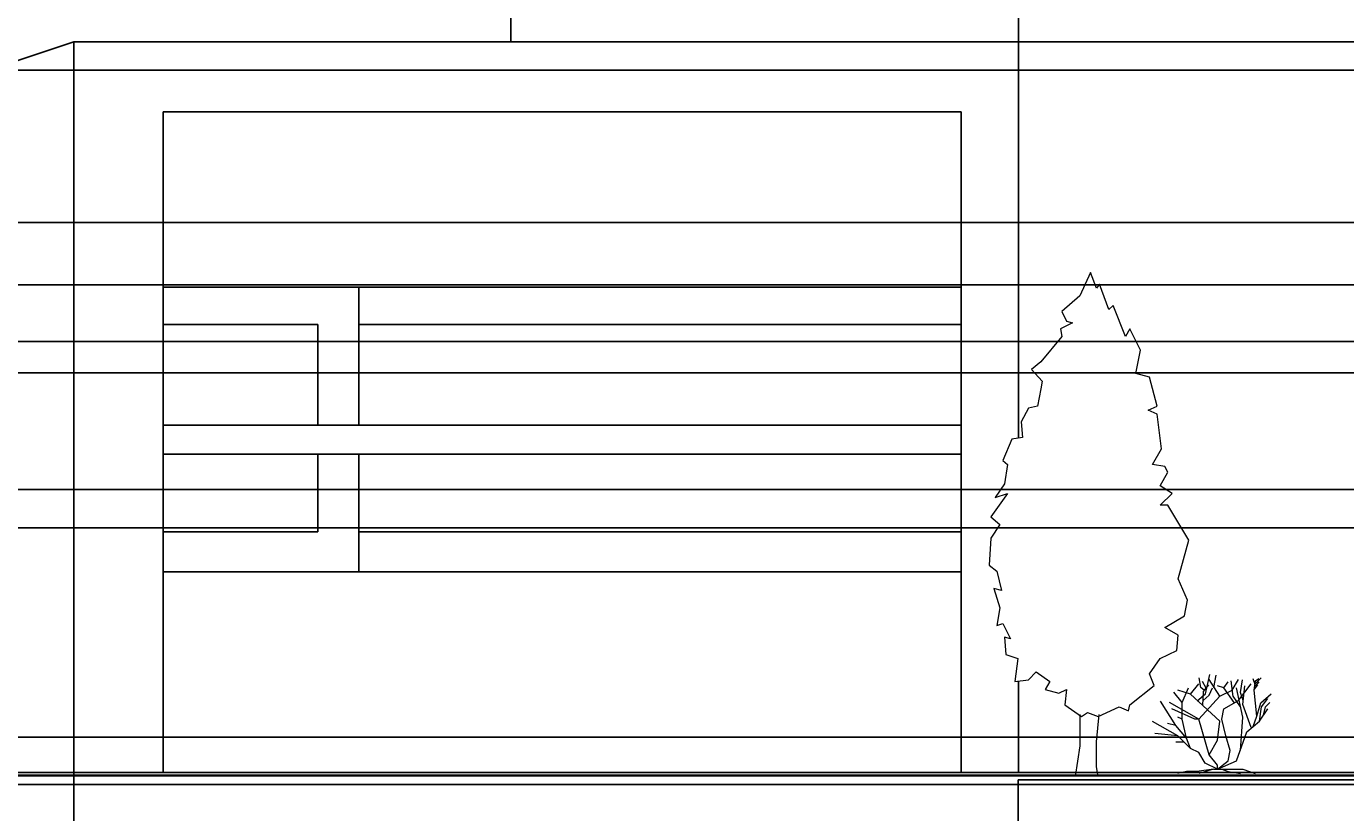
# Model space of a CAD drawing. Units: inches. Extents: x -32109 to 33221, y -19197 to 7608.
# Tile 21 of 25: x 15375 to 19011, y -2226 to -59. Entities that reach past the tile are written whole.
import ezdxf

# ---------------------------------------------------------------- set-up
doc = ezdxf.new("R2010")
doc.units = ezdxf.units.IN
doc.header["$MEASUREMENT"] = 0
for name, color, linetype, lineweight in [('A-ANNO-DIMS', 2, 'Continuous', 18), ('A-ELEV', 7, 'Continuous', 25), ('L-PLNT', 3, 'Continuous', 13)]:
    doc.layers.add(name, color=color, linetype=linetype, lineweight=lineweight)
doc.styles.get("Standard").update_dxf_attribs({"font": 'arial.ttf'})
doc.dimstyles.get("Standard").update_dxf_attribs({"dimtxt": 0.18, "dimasz": 0.18, "dimexe": 0.18, "dimexo": 0.0625, "dimgap": 0.09, "dimtad": 0, "dimtih": 1, "dimtoh": 1, "dimdec": 4, "dimzin": 0, "dimdsep": 46, "dimtxsty": 'Standard', "dimcen": 0.09, "dimadec": 0, "dimazin": 0, "dimtfac": 1, "dimtdec": 4, "dimtofl": 0, "dimtmove": 0, "dimatfit": 3, "dimfxl": 1, "dimtolj": 1, "dimtzin": 0, "dimarcsym": 0})

# ---------------------------------------------------------------- blocks, each defined once
blk = doc.blocks.new('*U2')
blk.add_lwpolyline([(-2.754, 191.699), (-6.78, 182.851), (-13.682, 176.953), (-11.956, 173.266), (-9.656, 172.529), (-14.257, 170.317), (-13.682, 167.368), (-21.733, 157.783), (-25.184, 154.834), (-21.158, 150.41), (-21.733, 147.461), (-22.884, 140.825), (-26.334, 140.087), (-29.21, 134.926), (-28.635, 129.028), (-32.661, 128.291), (-36.111, 120.18), (-34.386, 118.706), (-35.536, 111.333), (-38.987, 106.171), (-34.386, 107.646), (-40.712, 98.798), (-37.261, 95.849), (-40.712, 90.688), (-41.287, 80.366), (-38.412, 78.154), (-36.686, 70.781), (-39.562, 71.518), (-37.261, 64.145), (-38.412, 57.509), (-36.111, 58.247), (-33.236, 52.348), (-35.536, 53.086), (-34.961, 46.45), (-30.36, 44.975), (-31.51, 36.128), (-26.334, 36.865), (-23.459, 39.814), (-18.283, 36.128), (-20.008, 33.178), (-14.832, 31.704), (-11.956, 33.178), (-12.531, 27.28), (-6.205, 22.856), (-3.905, 24.331), (0.121, 22.856), (8.173, 26.543), (11.624, 25.068), (12.199, 27.28), (21.4, 34.653), (19.675, 39.077), (23.701, 44.975), (30.027, 47.924), (30.602, 53.823), (25.426, 56.772), (32.903, 61.196), (34.053, 67.094), (30.602, 75.205), (34.628, 89.951), (26.576, 103.222), (23.701, 103.222), (28.302, 107.646), (23.701, 110.595), (26.576, 115.756), (25.426, 117.968), (20.825, 118.706), (24.276, 124.604), (22.551, 137.876), (19.1, 139.35), (22.551, 140.825), (19.675, 151.884), (14.499, 153.359), (16.224, 162.207), (12.199, 170.317), (10.473, 167.368), (5.872, 179.165), (4.147, 177.69), (0.696, 187.275), (-0.454, 185.8)], close=True)
for points in [[(-6.813, 23.669), (-6.813, 11.669), (-8.627, 0)], [(0.387, 23.669), (-0.576, 13.271), (-0.576, 3.686), (0, 0)]]:
    blk.add_lwpolyline(points)
blk = doc.blocks.new('*U3')
for p, q in [((-12.471, 19.775), (-12.898, 22.044)), ((-11.433, 18.289), (-10.457, 22.749)), ((-8.16, 17.76), (-10.56, 21.6)), ((-9.48, 19.775), (-8.992, 22.592)), ((-5.086, 17.741), (-5.513, 21.34)), ((-5.28, 19.2), (-3.84, 21.6)), ((-3.377, 18.602), (-2.888, 21.575)), ((-0.508, 21.888), (-0.081, 20.558)), ((-0.203, 19.149), (0.102, 21.34)), ((0.041, 20.714), (1.384, 22.044)), ((0.102, 21.34), (0.835, 21.888)), ((-16.8, 16.32), (-18.72, 18.72)), ((-14.88, 18.24), (-17.76, 19.2)), ((-16.8, 16.32), (-15.36, 19.68)), ((-14.88, 18.24), (-12.96, 20.64)), ((-8.16, 12), (-14.88, 18.24)), ((-13.325, 16.724), (-11.433, 18.289)), ((-11.677, 19.071), (-12.471, 19.775)), ((-11.28, 19.619), (-12.104, 21.184)), ((-12.043, 15.628), (-11.921, 18.836)), ((-11.921, 18.836), (-10.64, 20.401)), ((-10.579, 18.054), (-9.846, 19.697)), ((-7.2, 19.68), (-8.64, 20.16)), ((-8.16, 17.76), (-5.28, 19.2)), ((-7.2, 19.68), (-6.24, 21.12)), ((-4.8, 16.32), (-7.2, 19.68)), ((-2.88, 12.96), (-4.32, 19.68)), ((-3.84, 16.8), (-0.96, 20.64)), ((-2.766, 16.802), (-3.377, 18.602)), ((-2.88, 15.84), (-2.4, 20.16)), ((0.346, 13.203), (-0.203, 19.149)), ((-0.142, 19.384), (0.59, 20.401)), ((-0.02, 20.01), (0.896, 21.105)), ((1.323, 16.254), (3.642, 18.289)), ((-18.24, 11.04), (-21.755, 16.655)), ((-12.96, 12.48), (-19.68, 16.32)), ((-16.8, 12.48), (-16.8, 16.32)), ((-12.96, 12.48), (-8.16, 17.76)), ((-11.982, 16.802), (-10.579, 18.054)), ((-7.2, 14.88), (-3.84, 16.8)), ((-3.377, 15.315), (-5.086, 17.819)), ((-0.96, 10.56), (-2.88, 15.84)), ((0.346, 13.203), (1.323, 16.254)), ((0.96, 12), (1.44, 15.36)), ((1.44, 15.36), (2.88, 17.28)), ((1.92, 13.44), (2.4, 15.36)), ((2.4, 15.36), (3.36, 16.32)), ((-13.92, 12.48), (-19.2, 14.88)), ((-16.8, 12.48), (-17.76, 12.96)), ((-15.84, 8.16), (-16.8, 12.48)), ((-12.96, 12.48), (-13.92, 12.48)), ((-10.56, 4.32), (-12.96, 12.48)), ((-7.68, 12.48), (-7.2, 14.88)), ((-6.72, 8.64), (-7.68, 12.48)), ((-3.36, 5.28), (-2.88, 12.96)), ((-0.48, 10.8), (0.346, 13.203)), ((0.96, 12), (2.88, 14.88)), ((-17.76, 8.64), (-23.663, 11.961)), ((-17.76, 8.64), (-23.128, 9.222)), ((-18.24, 11.04), (-20.16, 11.52)), ((-15.84, 8.16), (-18.24, 11.04)), ((-8.64, 7.68), (-8.16, 12)), ((-4.32, 2.88), (-1.92, 9.6)), ((-1.92, 9.6), (0.96, 12)), ((-16.32, 7.2), (-18.24, 7.2)), ((-14.88, 5.76), (-17.76, 8.64)), ((-14.88, 5.76), (-15.84, 8.16)), ((-10.56, 4.32), (-8.64, 7.68)), ((-5.76, 5.28), (-6.72, 8.64)), ((-12.96, 4.8), (-14.88, 5.76)), ((-11.52, 2.4), (-12.96, 4.8)), ((-8.64, 1.92), (-10.56, 4.32)), ((-6.24, 2.88), (-5.76, 5.28)), ((-15.84, 0.48), (-17.76, 0)), ((-13.44, 0.48), (-15.84, 0.48)), ((-9.6, 0.96), (-13.44, 0.48)), ((-9.6, 0.96), (-12.96, 0)), ((-8.64, 0.96), (-11.52, 2.4)), ((-9.6, 0.96), (-7.68, 0.96)), ((-8.64, 0.96), (-4.32, 2.88)), ((-8.64, 0.96), (-6.24, 2.88)), ((-8.64, 0.96), (-8.64, 1.92)), ((-8.64, 0.96), (-2.88, 0.96)), ((-7.68, 0.96), (-6.24, 0.48)), ((-6.24, 0.48), (-3.36, 0)), ((-2.88, 0.96), (0, 0))]:
    blk.add_line(p, q)
blk = doc.blocks.new('*D10')
at = {"layer": 'A-ANNO-DIMS', "color": 0, "lineweight": -2, "transparency": 16777216}
for p, q in [((-18512.6, -110.2), (-18512.6, 5772)), ((-18512.5, 5771.8), (-202.1, 5771.8)), ((18109.1, 5771.8), (-201.2, 5771.8)), ((18109.3, -101.5), (18109.3, 5772))]:
    blk.add_line(p, q, dxfattribs=at)
at = {"layer": 'A-ANNO-DIMS', "color": 0, "transparency": 16777216}
for points in [[(-18512.5, 5771.9), (-18512.5, 5771.8), (-18512.6, 5771.8)], [(18109.1, 5771.9), (18109.1, 5771.8), (18109.3, 5771.8)]]:
    blk.add_solid(points, dxfattribs=at)
at = {"layer": 'Defpoints', "color": 0, "transparency": 16777216}
for p in [(18109.3, 5771.8), (18109.3, -101.6), (-18512.6, -110.2)]:
    blk.add_point(p, dxfattribs=at)
at = {"layer": 'A-ANNO-DIMS', "color": 0, "transparency": 16777216, "insert": (-201.7, 5771.8), "char_height": 0.18, "attachment_point": 5}
blk.add_mtext('\\A1;36622', dxfattribs=at)
blk = doc.blocks.new('*D11')
at = {"layer": 'A-ANNO-DIMS', "color": 0, "lineweight": -2, "transparency": 16777216}
for p, q in [((14509.6, 1705.2), (25710.6, 1705.2)), ((25710.5, 1705), (25710.5, -209.6)), ((25710.5, -2124.6), (25710.5, -210)), ((-18512.6, -2124.8), (25710.6, -2124.8))]:
    blk.add_line(p, q, dxfattribs=at)
at = {"layer": 'A-ANNO-DIMS', "color": 0, "transparency": 16777216}
for points in [[(25710.4, 1705), (25710.5, 1705), (25710.5, 1705.2)], [(25710.4, -2124.6), (25710.5, -2124.6), (25710.5, -2124.8)]]:
    blk.add_solid(points, dxfattribs=at)
at = {"layer": 'Defpoints', "color": 0, "transparency": 16777216}
for p in [(14509.6, 1705.2), (-18512.6, -2124.8), (25710.5, -2124.8)]:
    blk.add_point(p, dxfattribs=at)
at = {"layer": 'A-ANNO-DIMS', "color": 0, "transparency": 16777216, "insert": (25710.5, -209.8), "char_height": 0.18, "attachment_point": 5}
blk.add_mtext('\\A1;3830', dxfattribs=at)
blk = doc.blocks.new('*D53')
at = {"layer": 'A-ANNO-DIMS', "color": 0, "lineweight": -2, "transparency": 16777216}
for p, q in [((-9508.3, -179.7), (25710.6, -179.7)), ((25710.5, -179.9), (25710.5, -389.7)), ((25710.5, -600), (25710.5, -390.1)), ((-9508.3, -600.2), (25710.6, -600.2))]:
    blk.add_line(p, q, dxfattribs=at)
at = {"layer": 'A-ANNO-DIMS', "color": 0, "transparency": 16777216}
for points in [[(25710.4, -179.9), (25710.5, -179.9), (25710.5, -179.7)], [(25710.4, -600), (25710.5, -600), (25710.5, -600.2)]]:
    blk.add_solid(points, dxfattribs=at)
at = {"layer": 'Defpoints', "color": 0, "transparency": 16777216}
for p in [(-9508.3, -179.7), (-9508.3, -600.2), (25710.5, -600.2)]:
    blk.add_point(p, dxfattribs=at)
at = {"layer": 'A-ANNO-DIMS', "color": 0, "transparency": 16777216, "insert": (25710.5, -389.9), "char_height": 0.18, "attachment_point": 5}
blk.add_mtext('\\A1;420.5', dxfattribs=at)
blk = doc.blocks.new('*D54')
at = {"layer": 'A-ANNO-DIMS', "color": 0, "lineweight": -2, "transparency": 16777216}
for p, q in [((-9508.3, -600.2), (25710.6, -600.2)), ((25710.5, -600.3), (25710.5, -806.8)), ((25710.5, -1013.7), (25710.5, -807.2)), ((-9508.3, -1013.9), (25710.6, -1013.9))]:
    blk.add_line(p, q, dxfattribs=at)
at = {"layer": 'A-ANNO-DIMS', "color": 0, "transparency": 16777216}
for points in [[(25710.4, -600.3), (25710.5, -600.3), (25710.5, -600.2)], [(25710.4, -1013.7), (25710.5, -1013.7), (25710.5, -1013.9)]]:
    blk.add_solid(points, dxfattribs=at)
at = {"layer": 'Defpoints', "color": 0, "transparency": 16777216}
for p in [(-9508.3, -600.2), (-9508.3, -1013.9), (25710.5, -1013.9)]:
    blk.add_point(p, dxfattribs=at)
at = {"layer": 'A-ANNO-DIMS', "color": 0, "transparency": 16777216, "insert": (25710.5, -807), "char_height": 0.18, "attachment_point": 5}
blk.add_mtext('\\A1;413.7', dxfattribs=at)
blk = doc.blocks.new('*D55')
at = {"layer": 'A-ANNO-DIMS', "color": 0, "lineweight": -2, "transparency": 16777216}
for p, q in [((-9508.3, -1013.9), (25710.6, -1013.9)), ((25710.5, -1014.1), (25710.5, -1227.7)), ((25710.5, -1441.6), (25710.5, -1228)), ((-9508.3, -1441.8), (25710.6, -1441.8))]:
    blk.add_line(p, q, dxfattribs=at)
at = {"layer": 'A-ANNO-DIMS', "color": 0, "transparency": 16777216}
for points in [[(25710.4, -1014.1), (25710.5, -1014.1), (25710.5, -1013.9)], [(25710.4, -1441.6), (25710.5, -1441.6), (25710.5, -1441.8)]]:
    blk.add_solid(points, dxfattribs=at)
at = {"layer": 'Defpoints', "color": 0, "transparency": 16777216}
for p in [(-9508.3, -1013.9), (-9508.3, -1441.8), (25710.5, -1441.8)]:
    blk.add_point(p, dxfattribs=at)
at = {"layer": 'A-ANNO-DIMS', "color": 0, "transparency": 16777216, "insert": (25710.5, -1227.9), "char_height": 0.18, "attachment_point": 5}
blk.add_mtext('\\A1;427.9', dxfattribs=at)
blk = doc.blocks.new('*D56')
at = {"layer": 'A-ANNO-DIMS', "color": 0, "lineweight": -2, "transparency": 16777216}
for p, q in [((-9508.3, -1441.8), (25710.6, -1441.8)), ((25710.5, -1442), (25710.5, -1730.1)), ((25710.5, -2018.6), (25710.5, -1730.5)), ((-9508.3, -2018.8), (25710.6, -2018.8))]:
    blk.add_line(p, q, dxfattribs=at)
at = {"layer": 'A-ANNO-DIMS', "color": 0, "transparency": 16777216}
for points in [[(25710.4, -1442), (25710.5, -1442), (25710.5, -1441.8)], [(25710.4, -2018.6), (25710.5, -2018.6), (25710.5, -2018.8)]]:
    blk.add_solid(points, dxfattribs=at)
at = {"layer": 'Defpoints', "color": 0, "transparency": 16777216}
for p in [(-9508.3, -1441.8), (-9508.3, -2018.8), (25710.5, -2018.8)]:
    blk.add_point(p, dxfattribs=at)
at = {"layer": 'A-ANNO-DIMS', "color": 0, "transparency": 16777216, "insert": (25710.5, -1730.3), "char_height": 0.18, "attachment_point": 5}
blk.add_mtext('\\A1;576.9', dxfattribs=at)
blk = doc.blocks.new('*D64')
at = {"layer": 'A-ANNO-DIMS', "color": 0, "lineweight": -2, "transparency": 16777216}
for p, q in [((14509.6, 1705.1), (14509.6, -5429.7)), ((15505.7, -101.7), (15505.7, -5429.7)), ((14509.7, -5429.6), (15007.3, -5429.6)), ((15505.6, -5429.6), (15008, -5429.6))]:
    blk.add_line(p, q, dxfattribs=at)
at = {"layer": 'A-ANNO-DIMS', "color": 0, "transparency": 16777216}
for points in [[(14509.7, -5429.5), (14509.7, -5429.6), (14509.6, -5429.6)], [(15505.6, -5429.5), (15505.6, -5429.6), (15505.7, -5429.6)]]:
    blk.add_solid(points, dxfattribs=at)
at = {"layer": 'Defpoints', "color": 0, "transparency": 16777216}
for p in [(14509.6, 1705.2), (15505.7, -101.6), (15505.7, -5429.6)]:
    blk.add_point(p, dxfattribs=at)
at = {"layer": 'A-ANNO-DIMS', "color": 0, "transparency": 16777216, "insert": (15007.6, -5429.6), "char_height": 0.18, "attachment_point": 5}
blk.add_mtext('\\A1;996.2', dxfattribs=at)
blk = doc.blocks.new('*D65')
at = {"layer": 'A-ANNO-DIMS', "color": 0, "lineweight": -2, "transparency": 16777216}
for p, q in [((15505.7, -101.7), (15505.7, -5429.7)), ((18108.4, -2136.1), (18108.4, -5429.7)), ((15505.9, -5429.6), (16806.6, -5429.6)), ((18108.2, -5429.6), (16807.5, -5429.6))]:
    blk.add_line(p, q, dxfattribs=at)
at = {"layer": 'A-ANNO-DIMS', "color": 0, "transparency": 16777216}
for points in [[(15505.9, -5429.5), (15505.9, -5429.6), (15505.7, -5429.6)], [(18108.2, -5429.5), (18108.2, -5429.6), (18108.4, -5429.6)]]:
    blk.add_solid(points, dxfattribs=at)
at = {"layer": 'Defpoints', "color": 0, "transparency": 16777216}
for p in [(15505.7, -101.6), (18108.4, -2136), (18108.4, -5429.6)]:
    blk.add_point(p, dxfattribs=at)
at = {"layer": 'A-ANNO-DIMS', "color": 0, "transparency": 16777216, "insert": (16807.1, -5429.6), "char_height": 0.18, "attachment_point": 5}
blk.add_mtext('\\A1;2602.6', dxfattribs=at)
blk = doc.blocks.new('*D67')
at = {"layer": 'A-ANNO-DIMS', "color": 0, "lineweight": -2, "transparency": 16777216}
for p, q in [((1645.9, 851.2), (25710.6, 851.2)), ((25710.5, 851), (25710.5, -632.3)), ((25710.5, -2116), (25710.5, -632.7)), ((1588.2, -2116.1), (25710.6, -2116.1))]:
    blk.add_line(p, q, dxfattribs=at)
at = {"layer": 'A-ANNO-DIMS', "color": 0, "transparency": 16777216}
for points in [[(25710.4, 851), (25710.5, 851), (25710.5, 851.2)], [(25710.4, -2116), (25710.5, -2116), (25710.5, -2116.1)]]:
    blk.add_solid(points, dxfattribs=at)
at = {"layer": 'Defpoints', "color": 0, "transparency": 16777216}
for p in [(1645.8, 851.2), (1588.2, -2116.1), (25710.5, -2116.1)]:
    blk.add_point(p, dxfattribs=at)
at = {"layer": 'A-ANNO-DIMS', "color": 0, "transparency": 16777216, "insert": (25710.5, -632.5), "char_height": 0.18, "attachment_point": 5}
blk.add_mtext('\\A1;2967.4', dxfattribs=at)
blk = doc.blocks.new('*D68')
at = {"layer": 'A-ANNO-DIMS', "color": 0, "lineweight": -2, "transparency": 16777216}
for p, q in [((4084.1, -927.5), (25710.6, -927.5)), ((25710.5, -927.7), (25710.5, -1521.6)), ((25710.5, -2116), (25710.5, -1522)), ((4084.1, -2116.1), (25710.6, -2116.1))]:
    blk.add_line(p, q, dxfattribs=at)
at = {"layer": 'A-ANNO-DIMS', "color": 0, "transparency": 16777216}
for points in [[(25710.4, -927.7), (25710.5, -927.7), (25710.5, -927.5)], [(25710.4, -2116), (25710.5, -2116), (25710.5, -2116.1)]]:
    blk.add_solid(points, dxfattribs=at)
at = {"layer": 'Defpoints', "color": 0, "transparency": 16777216}
for p in [(4084, -927.5), (4084, -2116.1), (25710.5, -2116.1)]:
    blk.add_point(p, dxfattribs=at)
at = {"layer": 'A-ANNO-DIMS', "color": 0, "transparency": 16777216, "insert": (25710.5, -1521.8), "char_height": 0.18, "attachment_point": 5}
blk.add_mtext('\\A1;1188.7', dxfattribs=at)
blk = doc.blocks.new('*D69')
at = {"layer": 'A-ANNO-DIMS', "color": 0, "lineweight": -2, "transparency": 16777216}
for p, q in [((5273.8, 1298.7), (25710.6, 1298.7)), ((25710.5, 1298.5), (25710.5, -411.9)), ((25710.5, -2122.6), (25710.5, -412.2)), ((5279.3, -2122.7), (25710.6, -2122.7))]:
    blk.add_line(p, q, dxfattribs=at)
at = {"layer": 'A-ANNO-DIMS', "color": 0, "transparency": 16777216}
for points in [[(25710.4, 1298.5), (25710.5, 1298.5), (25710.5, 1298.7)], [(25710.4, -2122.6), (25710.5, -2122.6), (25710.5, -2122.7)]]:
    blk.add_solid(points, dxfattribs=at)
at = {"layer": 'Defpoints', "color": 0, "transparency": 16777216}
for p in [(5273.7, 1298.7), (5279.3, -2122.7), (25710.5, -2122.7)]:
    blk.add_point(p, dxfattribs=at)
at = {"layer": 'A-ANNO-DIMS', "color": 0, "transparency": 16777216, "insert": (25710.5, -412), "char_height": 0.18, "attachment_point": 5}
blk.add_mtext('\\A1;3421.4', dxfattribs=at)
blk = doc.blocks.new('*D70')
at = {"layer": 'A-ANNO-DIMS', "color": 0, "lineweight": -2, "transparency": 16777216}
for p, q in [((8883.3, 57.8), (25710.6, 57.8)), ((25710.5, 57.6), (25710.5, -1045.1)), ((25710.5, -2148.2), (25710.5, -1045.5)), ((8832.4, -2148.4), (25710.6, -2148.4))]:
    blk.add_line(p, q, dxfattribs=at)
at = {"layer": 'A-ANNO-DIMS', "color": 0, "transparency": 16777216}
for points in [[(25710.4, 57.6), (25710.5, 57.6), (25710.5, 57.8)], [(25710.4, -2148.2), (25710.5, -2148.2), (25710.5, -2148.4)]]:
    blk.add_solid(points, dxfattribs=at)
at = {"layer": 'Defpoints', "color": 0, "transparency": 16777216}
for p in [(8883.2, 57.8), (8832.3, -2148.4), (25710.5, -2148.4)]:
    blk.add_point(p, dxfattribs=at)
at = {"layer": 'A-ANNO-DIMS', "color": 0, "transparency": 16777216, "insert": (25710.5, -1045.3), "char_height": 0.18, "attachment_point": 5}
blk.add_mtext('\\A1;2206', dxfattribs=at)
blk = doc.blocks.new('*D72')
at = {"layer": 'A-ANNO-DIMS', "color": 0, "lineweight": -2, "transparency": 16777216}
for p, q in [((11823.3, 107.7), (25710.6, 107.7)), ((25710.5, 107.6), (25710.5, -1004)), ((25710.5, -2116), (25710.5, -1004.4)), ((11383.7, -2116.1), (25710.6, -2116.1))]:
    blk.add_line(p, q, dxfattribs=at)
at = {"layer": 'A-ANNO-DIMS', "color": 0, "transparency": 16777216}
for points in [[(25710.4, 107.6), (25710.5, 107.6), (25710.5, 107.7)], [(25710.4, -2116), (25710.5, -2116), (25710.5, -2116.1)]]:
    blk.add_solid(points, dxfattribs=at)
at = {"layer": 'Defpoints', "color": 0, "transparency": 16777216}
for p in [(11823.2, 107.7), (11383.7, -2116.1), (25710.5, -2116.1)]:
    blk.add_point(p, dxfattribs=at)
at = {"layer": 'A-ANNO-DIMS', "color": 0, "transparency": 16777216, "insert": (25710.5, -1004.2), "char_height": 0.18, "attachment_point": 5}
blk.add_mtext('\\A1;2224', dxfattribs=at)
blk = doc.blocks.new('*D74')
at = {"layer": 'A-ANNO-DIMS', "color": 0, "lineweight": -2, "transparency": 16777216}
for p, q in [((15223.2, -771.9), (25710.6, -771.9)), ((25710.5, -772.1), (25710.5, -1053.6)), ((25710.5, -1335.5), (25710.5, -1054)), ((15223.2, -1335.7), (25710.6, -1335.7))]:
    blk.add_line(p, q, dxfattribs=at)
at = {"layer": 'A-ANNO-DIMS', "color": 0, "transparency": 16777216}
for points in [[(25710.4, -772.1), (25710.5, -772.1), (25710.5, -771.9)], [(25710.4, -1335.5), (25710.5, -1335.5), (25710.5, -1335.7)]]:
    blk.add_solid(points, dxfattribs=at)
at = {"layer": 'Defpoints', "color": 0, "transparency": 16777216}
for p in [(15223.2, -771.9), (15223.2, -1335.7), (25710.5, -1335.7)]:
    blk.add_point(p, dxfattribs=at)
at = {"layer": 'A-ANNO-DIMS', "color": 0, "transparency": 16777216, "insert": (25710.5, -1053.8), "char_height": 0.18, "attachment_point": 5}
blk.add_mtext('\\A1;563.8', dxfattribs=at)
blk = doc.blocks.new('*D76')
at = {"layer": 'A-ANNO-DIMS', "color": 0, "lineweight": -2, "transparency": 16777216}
for p, q in [((16709.9, 963.7), (25710.6, 963.7)), ((25710.5, 963.5), (25710.5, 431.2)), ((25710.5, -101.4), (25710.5, 430.9)), ((15505.8, -101.6), (25710.6, -101.6))]:
    blk.add_line(p, q, dxfattribs=at)
at = {"layer": 'A-ANNO-DIMS', "color": 0, "transparency": 16777216}
for points in [[(25710.4, 963.5), (25710.5, 963.5), (25710.5, 963.7)], [(25710.4, -101.4), (25710.5, -101.4), (25710.5, -101.6)]]:
    blk.add_solid(points, dxfattribs=at)
at = {"layer": 'Defpoints', "color": 0, "transparency": 16777216}
for p in [(16709.8, 963.7), (15505.7, -101.6), (25710.5, -101.6)]:
    blk.add_point(p, dxfattribs=at)
at = {"layer": 'A-ANNO-DIMS', "color": 0, "transparency": 16777216, "insert": (25710.5, 431.1), "char_height": 0.18, "attachment_point": 5}
blk.add_mtext('\\A1;1065.3', dxfattribs=at)
blk = doc.blocks.new('*D77')
at = {"layer": 'A-ANNO-DIMS', "color": 0, "lineweight": -2, "transparency": 16777216}
for p, q in [((18109.4, -101.6), (25710.6, -101.6)), ((25710.5, -101.8), (25710.5, -1118.6)), ((25710.5, -2135.8), (25710.5, -1119)), ((18108.4, -2136), (25710.6, -2136))]:
    blk.add_line(p, q, dxfattribs=at)
at = {"layer": 'A-ANNO-DIMS', "color": 0, "transparency": 16777216}
for points in [[(25710.4, -101.8), (25710.5, -101.8), (25710.5, -101.6)], [(25710.4, -2135.8), (25710.5, -2135.8), (25710.5, -2136)]]:
    blk.add_solid(points, dxfattribs=at)
at = {"layer": 'Defpoints', "color": 0, "transparency": 16777216}
for p in [(18109.3, -101.6), (18108.4, -2136), (25710.5, -2136)]:
    blk.add_point(p, dxfattribs=at)
at = {"layer": 'A-ANNO-DIMS', "color": 0, "transparency": 16777216, "insert": (25710.5, -1118.8), "char_height": 0.18, "attachment_point": 5}
blk.add_mtext('\\A1;2034.4', dxfattribs=at)

msp = doc.modelspace()

# ---------------------------------------------------------------- linework, layer by layer
at = {"layer": 'A-ELEV'}
for p, q in [((16709.825, 963.73), (16709.825, -101.6)), ((15505.744, -101.6), (14786.396, -341.579)), ((16709.825, -101.6), (15505.744, -101.6)), ((15505.744, -101.6), (15505.744, -2116.149)), ((16709.825, -101.6), (18109.317, -101.6)), ((18109.317, -101.6), (18109.317, -1194.086)), ((17951.347, -294.982), (15751.964, -294.982)), ((15751.964, -294.982), (15751.964, -2116.149)), ((15751.964, -294.982), (17951.347, -294.982)), ((17951.347, -2116.149), (17951.347, -294.982)), ((15751.964, -777.783), (17951.347, -777.783)), ((16290.918, -777.783), (16290.918, -1158.687)), ((15751.964, -881.239), (16177.923, -881.239)), ((16177.923, -881.239), (16177.923, -1158.687)), ((16290.918, -881.239), (17951.347, -881.239)), ((15751.964, -1158.687), (17951.347, -1158.687)), ((15751.964, -1238.629), (17951.347, -1238.629)), ((16177.923, -1238.629), (16177.923, -1452.503)), ((16290.918, -1238.629), (16290.918, -1563.103)), ((15751.964, -1452.503), (16177.923, -1452.503)), ((16290.918, -1452.503), (17951.347, -1452.503)), ((15751.964, -1563.103), (17951.347, -1563.103)), ((18109.317, -1863.915), (18109.317, -2116.149)), ((9873.793, -2116.149), (23260.469, -2116.149))]:
    msp.add_line(p, q, dxfattribs=at)

# ---------------------------------------------------------------- block references
at = {"layer": 'L-PLNT'}
for name, p, xscale, yscale, zscale in [('*U2', (18328.073, -2127.104), 7.247071498988421, 7.247071498988421, 7.247071498988421), ('*U3', (18761.791, -2118.431), 11.97885450539613, 11.97885450539613, 11.97885450539613)]:
    msp.add_blockref(name, p, dxfattribs=dict(at, xscale=xscale, yscale=yscale, zscale=zscale))

# ---------------------------------------------------------------- dimensions: what is measured, and where the dimension line sits
at = {"layer": 'A-ANNO-DIMS'}
for base, p1, p2, override, picture, middle in [((18109.317, 5771.835), (-18512.647, -110.242), (18109.317, -101.6), {"dimdec": 0, "dimlfac": 1, "dimrnd": 0, "dimzin": 0, "dimdsep": 46, "dimlunit": 2}, '*D10', (-201.665, 5771.835)), ((15505.744, -5429.555), (14509.55, 1705.162), (15505.744, -101.6), {"dimdec": 1, "dimlfac": 1, "dimrnd": 0, "dimzin": 0, "dimdsep": 46, "dimlunit": 2}, '*D64', (15007.647, -5429.555)), ((18108.369, -5429.555), (15505.744, -101.6), (18108.369, -2136.004), {"dimdec": 1, "dimlfac": 1, "dimrnd": 0, "dimzin": 0, "dimdsep": 46, "dimlunit": 2}, '*D65', (16807.057, -5429.555))]:
    dim = msp.add_linear_dim(base=base, p1=p1, p2=p2, dimstyle='Standard', override=override, dxfattribs=at)
    dim.commit()
    dim.dimension.update_dxf_attribs({"geometry": picture, "text_midpoint": middle})
for base, p1, p2, override, picture, middle in [((25710.469, -2124.791), (14509.55, 1705.162), (-18512.647, -2124.791), {"dimdec": 0, "dimlfac": 1, "dimrnd": 0, "dimzin": 0, "dimdsep": 46, "dimlunit": 2}, '*D11', (25710.469, -209.814)), ((25710.469, -2122.749), (5273.749, 1298.671), (5279.264, -2122.749), {"dimdec": 1, "dimlfac": 1, "dimrnd": 0, "dimzin": 0, "dimdsep": 46, "dimlunit": 2}, '*D69', (25710.469, -412.039)), ((25710.469, -101.6), (16709.825, 963.73), (15505.744, -101.6), {"dimdec": 1, "dimlfac": 1, "dimrnd": 0, "dimzin": 0, "dimdsep": 46, "dimlunit": 2}, '*D76', (25710.469, 431.065)), ((25710.469, -2116.149), (1645.845, 851.205), (1588.181, -2116.149), {"dimdec": 1, "dimlfac": 1, "dimrnd": 0, "dimzin": 0, "dimdsep": 46, "dimlunit": 2}, '*D67', (25710.469, -632.472)), ((25710.469, -2116.149), (11823.239, 107.745), (11383.682, -2116.149), {"dimdec": 0, "dimlfac": 1, "dimrnd": 0, "dimzin": 0, "dimdsep": 46, "dimlunit": 2}, '*D72', (25710.469, -1004.202)), ((25710.469, -2148.367), (8883.215, 57.799), (8832.289, -2148.367), {"dimdec": 0, "dimlfac": 1, "dimrnd": 0, "dimzin": 0, "dimdsep": 46, "dimlunit": 2}, '*D70', (25710.469, -1045.284)), ((25710.469, -2136.004), (18109.317, -101.6), (18108.369, -2136.004), {"dimdec": 1, "dimlfac": 1, "dimrnd": 0, "dimzin": 0, "dimdsep": 46, "dimlunit": 2}, '*D77', (25710.469, -1118.802)), ((25710.469, -600.154), (-9508.333, -179.679), (-9508.333, -600.154), {"dimdec": 1, "dimlfac": 1, "dimrnd": 0, "dimzin": 0, "dimdsep": 46, "dimlunit": 2}, '*D53', (25710.469, -389.916)), ((25710.469, -1013.888), (-9508.333, -600.154), (-9508.333, -1013.888), {"dimdec": 1, "dimlfac": 1, "dimrnd": 0, "dimzin": 0, "dimdsep": 46, "dimlunit": 2}, '*D54', (25710.469, -807.021)), ((25710.469, -1335.677), (15223.17, -771.886), (15223.17, -1335.677), {"dimdec": 1, "dimlfac": 1, "dimrnd": 0, "dimzin": 0, "dimdsep": 46, "dimlunit": 2}, '*D74', (25710.469, -1053.781)), ((25710.469, -2116.149), (4083.997, -927.479), (4083.997, -2116.149), {"dimdec": 1, "dimlfac": 1, "dimrnd": 0, "dimzin": 0, "dimdsep": 46, "dimlunit": 2}, '*D68', (25710.469, -1521.814)), ((25710.469, -1441.815), (-9508.333, -1013.888), (-9508.333, -1441.815), {"dimdec": 1, "dimlfac": 1, "dimrnd": 0, "dimzin": 0, "dimdsep": 46, "dimlunit": 2}, '*D55', (25710.469, -1227.851)), ((25710.469, -2018.754), (-9508.333, -1441.815), (-9508.333, -2018.754), {"dimdec": 1, "dimlfac": 1, "dimrnd": 0, "dimzin": 0, "dimdsep": 46, "dimlunit": 2}, '*D56', (25710.469, -1730.285))]:
    dim = msp.add_linear_dim(base=base, p1=p1, p2=p2, angle=90, dimstyle='Standard', override=override, dxfattribs=at)
    dim.commit()
    dim.dimension.update_dxf_attribs({"geometry": picture, "text_midpoint": middle})

doc.saveas('drawing.dxf')
